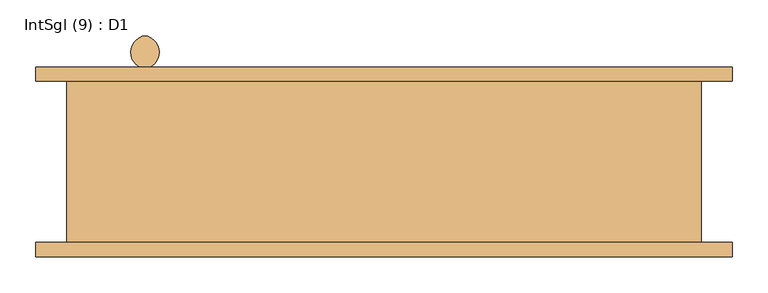
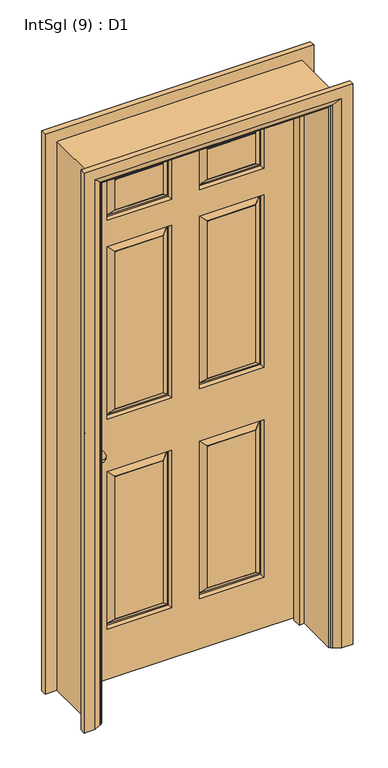
"""IFC4 building model written with IfcOpenShell, lengths in millimetres: door geometry, IntSgl (9) : D1."""

from ifc_helpers import new_model, si_unit, point, frame, origin, place, context, project, spatial, polyline, circle_curve, ellipse_curve, trimmed, outline, extrude, faceted_brep, source, transform, mapped, element, save
from ifc_brep_helpers import plane_surface, cylinder_surface, revolved_surface, advanced_brep


def intsgl_9_d1_c400c9dc(model_context):
    return source(origin(), model_context, "Body", "SolidModel", [
        advanced_brep(
        [(-328.0, 55.5, 900.0), (-333.0, 11.062589, 900.0), (-338.0, 55.5, 900.0), (-338.0, 70.5, 900.0), (-328.0, 70.5, 900.0), (-353.0, 74.5, 900.0), (-313.0, 74.5, 900.0), (-353.0, 70.5, 900.0), (-313.0, 70.5, 900.0)],
        [
            (0, 1, circle_curve(frame((-336.1884862, 33.9213505, 900.0), z_axis=(0.0, 0.0, -1.0), x_axis=(0.0, 1.0, 0.0)), 23.0800654)),
            (1, 2, circle_curve(frame((-329.8115138, 33.9213505, 900.0), z_axis=(0.0, 0.0, -1.0), x_axis=(0.0, 1.0, 0.0)), 23.0800654)),
            (2, 0, circle_curve(frame((-333.0, 55.5, 900.0), z_axis=(0.0, -1.0, 0.0), x_axis=(-1.0, 0.0, 0.0)), 5.0)),
            (0, 2, circle_curve(frame((-333.0, 55.5, 900.0), z_axis=(0.0, -1.0, 0.0), x_axis=(-1.0, 0.0, 0.0)), 5.0)),
            (2, 3),
            (3, 4, circle_curve(frame((-333.0, 70.5, 900.0), z_axis=(0.0, -1.0, 0.0), x_axis=(-1.0, 0.0, 0.0)), 5.0)),
            (4, 0),
            (4, 3, circle_curve(frame((-333.0, 70.5, 900.0), z_axis=(0.0, -1.0, 0.0), x_axis=(-1.0, 0.0, 0.0)), 5.0)),
            (5, 6, circle_curve(frame((-333.0, 74.5, 900.0), z_axis=(0.0, 1.0, 0.0), x_axis=(1.0, 0.0, 0.0)), 20.0)),
            (6, 5, circle_curve(frame((-333.0, 74.5, 900.0), z_axis=(0.0, 1.0, 0.0), x_axis=(1.0, 0.0, 0.0)), 20.0)),
            (7, 8, circle_curve(frame((-333.0, 70.5, 900.0), z_axis=(0.0, -1.0, 0.0), x_axis=(1.0, 0.0, 0.0)), 20.0)),
            (8, 7, circle_curve(frame((-333.0, 70.5, 900.0), z_axis=(0.0, -1.0, 0.0), x_axis=(1.0, 0.0, 0.0)), 20.0)),
            (6, 8),
            (7, 5),
        ],
        [
            revolved_surface(trimmed(ellipse_curve(frame((-329.8115138, 33.9213505, 900.0), z_axis=(0.0, 0.0, -1.0), x_axis=(0.0, 1.0, 0.0)), 23.0800654, 23.0800654), [point((-333.0, 11.062589, 900.0))], [point((-338.0, 55.5, 900.0))], True, "CARTESIAN"), (-333.0, 70.5, 900.0), (0.0, 1.0, 0.0)),
            cylinder_surface(frame((-333.0, 70.5, 900.0), z_axis=(0.0, 1.0, 0.0), x_axis=(-1.0, 0.0, 0.0)), 5.0),
            plane_surface(frame((-313.0, 74.5, 900.0), z_axis=(0.0, 1.0, 0.0), x_axis=(0.0, 0.0, 1.0))),
            plane_surface(frame((-313.0, 70.5, 900.0), z_axis=(0.0, -1.0, 0.0), x_axis=(0.0, 0.0, -1.0))),
            cylinder_surface(frame((-333.0, 70.5, 900.0), z_axis=(0.0, 1.0, 0.0), x_axis=(1.0, 0.0, 0.0)), 20.0),
        ],
        [
            (0, [[1, 2, 3]]),
            (0, [[-1, 4, -2]]),
            (1, [[5, 6, 7, -3]]),
            (1, [[-7, 8, -5, -4]]),
            (2, [[9, 10]]),
            (3, [[11, 12], [-8, -6]]),
            (4, [[13, -11, 14, -10]]),
            (4, [[-14, -12, -13, -9]]),
        ],
    ),
        advanced_brep(
        [(-328.0, 131.5, 900.0), (-338.0, 131.5, 900.0), (-333.0, 175.937411, 900.0), (-328.0, 116.5, 900.0), (-338.0, 116.5, 900.0), (-353.0, 112.5, 900.0), (-313.0, 112.5, 900.0), (-353.0, 116.5, 900.0), (-313.0, 116.5, 900.0)],
        [
            (0, 1, circle_curve(frame((-333.0, 131.5, 900.0), z_axis=(0.0, 1.0, 0.0), x_axis=(-1.0, 0.0, 0.0)), 5.0)),
            (1, 2, circle_curve(frame((-329.8115138, 153.0786495, 900.0), z_axis=(0.0, 0.0, -1.0), x_axis=(0.0, -1.0, 0.0)), 23.0800654)),
            (2, 0, circle_curve(frame((-336.1884862, 153.0786495, 900.0), z_axis=(0.0, 0.0, -1.0), x_axis=(0.0, -1.0, 0.0)), 23.0800654)),
            (1, 0, circle_curve(frame((-333.0, 131.5, 900.0), z_axis=(0.0, 1.0, 0.0), x_axis=(-1.0, 0.0, 0.0)), 5.0)),
            (0, 3),
            (3, 4, circle_curve(frame((-333.0, 116.5, 900.0), z_axis=(0.0, 1.0, 0.0), x_axis=(-1.0, 0.0, 0.0)), 5.0)),
            (4, 1),
            (4, 3, circle_curve(frame((-333.0, 116.5, 900.0), z_axis=(0.0, 1.0, 0.0), x_axis=(-1.0, 0.0, 0.0)), 5.0)),
            (5, 6, circle_curve(frame((-333.0, 112.5, 900.0), z_axis=(0.0, -1.0, 0.0), x_axis=(1.0, 0.0, 0.0)), 20.0)),
            (6, 5, circle_curve(frame((-333.0, 112.5, 900.0), z_axis=(0.0, -1.0, 0.0), x_axis=(1.0, 0.0, 0.0)), 20.0)),
            (7, 8, circle_curve(frame((-333.0, 116.5, 900.0), z_axis=(0.0, 1.0, 0.0), x_axis=(1.0, 0.0, 0.0)), 20.0)),
            (8, 7, circle_curve(frame((-333.0, 116.5, 900.0), z_axis=(0.0, 1.0, 0.0), x_axis=(1.0, 0.0, 0.0)), 20.0)),
            (5, 7),
            (8, 6),
        ],
        [
            revolved_surface(trimmed(ellipse_curve(frame((-329.8115138, 153.0786495, 900.0), z_axis=(0.0, 0.0, 1.0), x_axis=(0.0, -1.0, 0.0)), 23.0800654, 23.0800654), [point((-333.0, 175.937411, 900.0))], [point((-338.0, 131.5, 900.0))], True, "CARTESIAN"), (-333.0, 116.5, 900.0), (0.0, -1.0, 0.0)),
            cylinder_surface(frame((-333.0, 116.5, 900.0), z_axis=(0.0, -1.0, 0.0), x_axis=(-1.0, 0.0, 0.0)), 5.0),
            plane_surface(frame((-313.0, 112.5, 900.0), z_axis=(0.0, -1.0, 0.0), x_axis=(0.0, 0.0, 1.0))),
            plane_surface(frame((-313.0, 116.5, 900.0), z_axis=(0.0, 1.0, 0.0), x_axis=(0.0, 0.0, -1.0))),
            cylinder_surface(frame((-333.0, 116.5, 900.0), z_axis=(0.0, -1.0, 0.0), x_axis=(1.0, 0.0, 0.0)), 20.0),
        ],
        [
            (0, [[1, 2, 3]]),
            (0, [[-2, 4, -3]]),
            (1, [[-1, 5, 6, 7]]),
            (1, [[-4, -7, 8, -5]]),
            (2, [[9, 10]]),
            (3, [[11, 12], [-6, -8]]),
            (4, [[-9, 13, -12, 14]]),
            (4, [[-10, -14, -11, -13]]),
        ],
    ),
        faceted_brep([(-408.0, 74.5, 2058.0), (-408.0, 74.5, 8.0), (408.0, 74.5, 8.0), (408.0, 74.5, 2058.0), (-50.0, 74.5, 800.0), (-50.0, 74.5, 200.0), (-283.0, 74.5, 200.0), (-283.0, 74.5, 800.0), (283.0, 74.5, 800.0), (283.0, 74.5, 200.0), (50.0, 74.5, 200.0), (50.0, 74.5, 800.0), (-50.0, 74.5, 1658.0), (-50.0, 74.5, 1000.0), (-283.0, 74.5, 1000.0), (-283.0, 74.5, 1658.0), (283.0, 74.5, 1658.0), (283.0, 74.5, 1000.0), (50.0, 74.5, 1000.0), (50.0, 74.5, 1658.0), (-50.0, 74.5, 1933.0), (-50.0, 74.5, 1758.0), (-283.0, 74.5, 1758.0), (-283.0, 74.5, 1933.0), (283.0, 74.5, 1933.0), (283.0, 74.5, 1758.0), (50.0, 74.5, 1758.0), (50.0, 74.5, 1933.0), (-80.0, 74.5, 230.0), (-80.0, 74.5, 770.0), (-253.0, 74.5, 770.0), (-253.0, 74.5, 230.0), (253.0, 74.5, 230.0), (253.0, 74.5, 770.0), (80.0, 74.5, 770.0), (80.0, 74.5, 230.0), (-80.0, 74.5, 1030.0), (-80.0, 74.5, 1628.0), (-253.0, 74.5, 1628.0), (-253.0, 74.5, 1030.0), (253.0, 74.5, 1030.0), (253.0, 74.5, 1628.0), (80.0, 74.5, 1628.0), (80.0, 74.5, 1030.0), (-80.0, 74.5, 1788.0), (-80.0, 74.5, 1903.0), (-253.0, 74.5, 1903.0), (-253.0, 74.5, 1788.0), (253.0, 74.5, 1788.0), (253.0, 74.5, 1903.0), (80.0, 74.5, 1903.0), (80.0, 74.5, 1788.0), (-408.0, 112.5, 2058.0), (408.0, 112.5, 2058.0), (408.0, 112.5, 8.0), (-408.0, 112.5, 8.0), (50.0, 112.5, 800.0), (50.0, 112.5, 200.0), (283.0, 112.5, 200.0), (283.0, 112.5, 800.0), (-283.0, 112.5, 800.0), (-283.0, 112.5, 200.0), (-50.0, 112.5, 200.0), (-50.0, 112.5, 800.0), (50.0, 112.5, 1658.0), (50.0, 112.5, 1000.0), (283.0, 112.5, 1000.0), (283.0, 112.5, 1658.0), (-283.0, 112.5, 1658.0), (-283.0, 112.5, 1000.0), (-50.0, 112.5, 1000.0), (-50.0, 112.5, 1658.0), (50.0, 112.5, 1933.0), (50.0, 112.5, 1758.0), (283.0, 112.5, 1758.0), (283.0, 112.5, 1933.0), (-283.0, 112.5, 1933.0), (-283.0, 112.5, 1758.0), (-50.0, 112.5, 1758.0), (-50.0, 112.5, 1933.0), (80.0, 112.5, 230.0), (80.0, 112.5, 770.0), (253.0, 112.5, 770.0), (253.0, 112.5, 230.0), (-253.0, 112.5, 230.0), (-253.0, 112.5, 770.0), (-80.0, 112.5, 770.0), (-80.0, 112.5, 230.0), (80.0, 112.5, 1030.0), (80.0, 112.5, 1628.0), (253.0, 112.5, 1628.0), (253.0, 112.5, 1030.0), (-253.0, 112.5, 1030.0), (-253.0, 112.5, 1628.0), (-80.0, 112.5, 1628.0), (-80.0, 112.5, 1030.0), (80.0, 112.5, 1788.0), (80.0, 112.5, 1903.0), (253.0, 112.5, 1903.0), (253.0, 112.5, 1788.0), (-253.0, 112.5, 1788.0), (-253.0, 112.5, 1903.0), (-80.0, 112.5, 1903.0), (-80.0, 112.5, 1788.0), (80.0, 111.5, 230.0), (80.0, 111.5, 770.0), (58.0, 97.5, 208.0), (58.0, 97.5, 792.0), (78.0, 111.5, 772.0), (78.0, 111.5, 228.0), (53.0, 97.5, 797.0), (53.0, 97.5, 203.0), (253.0, 111.5, 770.0), (275.0, 97.5, 792.0), (255.0, 111.5, 772.0), (280.0, 97.5, 797.0), (253.0, 111.5, 230.0), (275.0, 97.5, 208.0), (255.0, 111.5, 228.0), (280.0, 97.5, 203.0), (-253.0, 111.5, 230.0), (-253.0, 111.5, 770.0), (-275.0, 97.5, 208.0), (-275.0, 97.5, 792.0), (-255.0, 111.5, 772.0), (-255.0, 111.5, 228.0), (-280.0, 97.5, 797.0), (-280.0, 97.5, 203.0), (-80.0, 111.5, 770.0), (-58.0, 97.5, 792.0), (-78.0, 111.5, 772.0), (-53.0, 97.5, 797.0), (-80.0, 111.5, 230.0), (-58.0, 97.5, 208.0), (-78.0, 111.5, 228.0), (-53.0, 97.5, 203.0), (80.0, 111.5, 1030.0), (80.0, 111.5, 1628.0), (58.0, 97.5, 1008.0), (58.0, 97.5, 1650.0), (78.0, 111.5, 1630.0), (78.0, 111.5, 1028.0), (53.0, 97.5, 1655.0), (53.0, 97.5, 1003.0), (253.0, 111.5, 1628.0), (275.0, 97.5, 1650.0), (255.0, 111.5, 1630.0), (280.0, 97.5, 1655.0), (253.0, 111.5, 1030.0), (275.0, 97.5, 1008.0), (255.0, 111.5, 1028.0), (280.0, 97.5, 1003.0), (-253.0, 111.5, 1030.0), (-253.0, 111.5, 1628.0), (-275.0, 97.5, 1008.0), (-275.0, 97.5, 1650.0), (-255.0, 111.5, 1630.0), (-255.0, 111.5, 1028.0), (-280.0, 97.5, 1655.0), (-280.0, 97.5, 1003.0), (-80.0, 111.5, 1628.0), (-58.0, 97.5, 1650.0), (-78.0, 111.5, 1630.0), (-53.0, 97.5, 1655.0), (-80.0, 111.5, 1030.0), (-58.0, 97.5, 1008.0), (-78.0, 111.5, 1028.0), (-53.0, 97.5, 1003.0), (80.0, 111.5, 1788.0), (80.0, 111.5, 1903.0), (58.0, 97.5, 1766.0), (58.0, 97.5, 1925.0), (78.0, 111.5, 1905.0), (78.0, 111.5, 1786.0), (53.0, 97.5, 1930.0), (53.0, 97.5, 1761.0), (253.0, 111.5, 1903.0), (275.0, 97.5, 1925.0), (255.0, 111.5, 1905.0), (280.0, 97.5, 1930.0), (253.0, 111.5, 1788.0), (275.0, 97.5, 1766.0), (255.0, 111.5, 1786.0), (280.0, 97.5, 1761.0), (-253.0, 111.5, 1788.0), (-253.0, 111.5, 1903.0), (-275.0, 97.5, 1766.0), (-275.0, 97.5, 1925.0), (-255.0, 111.5, 1905.0), (-255.0, 111.5, 1786.0), (-280.0, 97.5, 1930.0), (-280.0, 97.5, 1761.0), (-80.0, 111.5, 1903.0), (-58.0, 97.5, 1925.0), (-78.0, 111.5, 1905.0), (-53.0, 97.5, 1930.0), (-80.0, 111.5, 1788.0), (-58.0, 97.5, 1766.0), (-78.0, 111.5, 1786.0), (-53.0, 97.5, 1761.0), (-80.0, 75.5, 230.0), (-80.0, 75.5, 770.0), (-58.0, 89.5, 208.0), (-58.0, 89.5, 792.0), (-78.0, 75.5, 772.0), (-78.0, 75.5, 228.0), (-53.0, 89.5, 797.0), (-53.0, 89.5, 203.0), (-253.0, 75.5, 770.0), (-275.0, 89.5, 792.0), (-255.0, 75.5, 772.0), (-280.0, 89.5, 797.0), (-253.0, 75.5, 230.0), (-275.0, 89.5, 208.0), (-255.0, 75.5, 228.0), (-280.0, 89.5, 203.0), (253.0, 75.5, 230.0), (253.0, 75.5, 770.0), (275.0, 89.5, 208.0), (275.0, 89.5, 792.0), (255.0, 75.5, 772.0), (255.0, 75.5, 228.0), (280.0, 89.5, 797.0), (280.0, 89.5, 203.0), (80.0, 75.5, 770.0), (58.0, 89.5, 792.0), (78.0, 75.5, 772.0), (53.0, 89.5, 797.0), (80.0, 75.5, 230.0), (58.0, 89.5, 208.0), (78.0, 75.5, 228.0), (53.0, 89.5, 203.0), (-80.0, 75.5, 1030.0), (-80.0, 75.5, 1628.0), (-58.0, 89.5, 1008.0), (-58.0, 89.5, 1650.0), (-78.0, 75.5, 1630.0), (-78.0, 75.5, 1028.0), (-53.0, 89.5, 1655.0), (-53.0, 89.5, 1003.0), (-253.0, 75.5, 1628.0), (-275.0, 89.5, 1650.0), (-255.0, 75.5, 1630.0), (-280.0, 89.5, 1655.0), (-253.0, 75.5, 1030.0), (-275.0, 89.5, 1008.0), (-255.0, 75.5, 1028.0), (-280.0, 89.5, 1003.0), (253.0, 75.5, 1030.0), (253.0, 75.5, 1628.0), (275.0, 89.5, 1008.0), (275.0, 89.5, 1650.0), (255.0, 75.5, 1630.0), (255.0, 75.5, 1028.0), (280.0, 89.5, 1655.0), (280.0, 89.5, 1003.0), (80.0, 75.5, 1628.0), (58.0, 89.5, 1650.0), (78.0, 75.5, 1630.0), (53.0, 89.5, 1655.0), (80.0, 75.5, 1030.0), (58.0, 89.5, 1008.0), (78.0, 75.5, 1028.0), (53.0, 89.5, 1003.0), (-80.0, 75.5, 1788.0), (-80.0, 75.5, 1903.0), (-58.0, 89.5, 1766.0), (-58.0, 89.5, 1925.0), (-78.0, 75.5, 1905.0), (-78.0, 75.5, 1786.0), (-53.0, 89.5, 1930.0), (-53.0, 89.5, 1761.0), (-253.0, 75.5, 1903.0), (-275.0, 89.5, 1925.0), (-255.0, 75.5, 1905.0), (-280.0, 89.5, 1930.0), (-253.0, 75.5, 1788.0), (-275.0, 89.5, 1766.0), (-255.0, 75.5, 1786.0), (-280.0, 89.5, 1761.0), (253.0, 75.5, 1788.0), (253.0, 75.5, 1903.0), (275.0, 89.5, 1766.0), (275.0, 89.5, 1925.0), (255.0, 75.5, 1905.0), (255.0, 75.5, 1786.0), (280.0, 89.5, 1930.0), (280.0, 89.5, 1761.0), (80.0, 75.5, 1903.0), (58.0, 89.5, 1925.0), (78.0, 75.5, 1905.0), (53.0, 89.5, 1930.0), (80.0, 75.5, 1788.0), (58.0, 89.5, 1766.0), (78.0, 75.5, 1786.0), (53.0, 89.5, 1761.0)], [[[0, 1, 2, 3], [4, 5, 6, 7], [8, 9, 10, 11], [12, 13, 14, 15], [16, 17, 18, 19], [20, 21, 22, 23], [24, 25, 26, 27]], [[28, 29, 30, 31]], [[32, 33, 34, 35]], [[36, 37, 38, 39]], [[40, 41, 42, 43]], [[44, 45, 46, 47]], [[48, 49, 50, 51]], [[52, 53, 54, 55], [56, 57, 58, 59], [60, 61, 62, 63], [64, 65, 66, 67], [68, 69, 70, 71], [72, 73, 74, 75], [76, 77, 78, 79]], [[80, 81, 82, 83]], [[84, 85, 86, 87]], [[88, 89, 90, 91]], [[92, 93, 94, 95]], [[96, 97, 98, 99]], [[100, 101, 102, 103]], [[1, 0, 52, 55]], [[2, 1, 55, 54]], [[3, 2, 54, 53]], [[0, 3, 53, 52]], [[104, 105, 81, 80]], [[106, 107, 108, 109]], [[56, 110, 111, 57]], [[81, 105, 112, 82]], [[108, 107, 113, 114]], [[110, 56, 59, 115]], [[82, 112, 116, 83]], [[114, 113, 117, 118]], [[115, 59, 58, 119]], [[104, 80, 83, 116]], [[109, 108, 114, 118], [105, 104, 116, 112]], [[106, 109, 118, 117]], [[111, 110, 115, 119], [107, 106, 117, 113]], [[57, 111, 119, 58]], [[120, 121, 85, 84]], [[122, 123, 124, 125]], [[60, 126, 127, 61]], [[85, 121, 128, 86]], [[124, 123, 129, 130]], [[126, 60, 63, 131]], [[86, 128, 132, 87]], [[130, 129, 133, 134]], [[131, 63, 62, 135]], [[120, 84, 87, 132]], [[125, 124, 130, 134], [121, 120, 132, 128]], [[122, 125, 134, 133]], [[127, 126, 131, 135], [123, 122, 133, 129]], [[61, 127, 135, 62]], [[136, 137, 89, 88]], [[138, 139, 140, 141]], [[64, 142, 143, 65]], [[89, 137, 144, 90]], [[140, 139, 145, 146]], [[142, 64, 67, 147]], [[90, 144, 148, 91]], [[146, 145, 149, 150]], [[147, 67, 66, 151]], [[136, 88, 91, 148]], [[141, 140, 146, 150], [137, 136, 148, 144]], [[138, 141, 150, 149]], [[143, 142, 147, 151], [139, 138, 149, 145]], [[65, 143, 151, 66]], [[152, 153, 93, 92]], [[154, 155, 156, 157]], [[68, 158, 159, 69]], [[93, 153, 160, 94]], [[156, 155, 161, 162]], [[158, 68, 71, 163]], [[94, 160, 164, 95]], [[162, 161, 165, 166]], [[163, 71, 70, 167]], [[152, 92, 95, 164]], [[157, 156, 162, 166], [153, 152, 164, 160]], [[154, 157, 166, 165]], [[159, 158, 163, 167], [155, 154, 165, 161]], [[69, 159, 167, 70]], [[168, 169, 97, 96]], [[170, 171, 172, 173]], [[72, 174, 175, 73]], [[97, 169, 176, 98]], [[172, 171, 177, 178]], [[174, 72, 75, 179]], [[98, 176, 180, 99]], [[178, 177, 181, 182]], [[179, 75, 74, 183]], [[168, 96, 99, 180]], [[173, 172, 178, 182], [169, 168, 180, 176]], [[170, 173, 182, 181]], [[175, 174, 179, 183], [171, 170, 181, 177]], [[73, 175, 183, 74]], [[184, 185, 101, 100]], [[186, 187, 188, 189]], [[76, 190, 191, 77]], [[101, 185, 192, 102]], [[188, 187, 193, 194]], [[190, 76, 79, 195]], [[102, 192, 196, 103]], [[194, 193, 197, 198]], [[195, 79, 78, 199]], [[184, 100, 103, 196]], [[189, 188, 194, 198], [185, 184, 196, 192]], [[186, 189, 198, 197]], [[191, 190, 195, 199], [187, 186, 197, 193]], [[77, 191, 199, 78]], [[200, 201, 29, 28]], [[202, 203, 204, 205]], [[4, 206, 207, 5]], [[29, 201, 208, 30]], [[204, 203, 209, 210]], [[206, 4, 7, 211]], [[30, 208, 212, 31]], [[210, 209, 213, 214]], [[211, 7, 6, 215]], [[200, 28, 31, 212]], [[205, 204, 210, 214], [201, 200, 212, 208]], [[202, 205, 214, 213]], [[207, 206, 211, 215], [203, 202, 213, 209]], [[5, 207, 215, 6]], [[216, 217, 33, 32]], [[218, 219, 220, 221]], [[8, 222, 223, 9]], [[33, 217, 224, 34]], [[220, 219, 225, 226]], [[222, 8, 11, 227]], [[34, 224, 228, 35]], [[226, 225, 229, 230]], [[227, 11, 10, 231]], [[216, 32, 35, 228]], [[221, 220, 226, 230], [217, 216, 228, 224]], [[218, 221, 230, 229]], [[223, 222, 227, 231], [219, 218, 229, 225]], [[9, 223, 231, 10]], [[232, 233, 37, 36]], [[234, 235, 236, 237]], [[12, 238, 239, 13]], [[37, 233, 240, 38]], [[236, 235, 241, 242]], [[238, 12, 15, 243]], [[38, 240, 244, 39]], [[242, 241, 245, 246]], [[243, 15, 14, 247]], [[232, 36, 39, 244]], [[237, 236, 242, 246], [233, 232, 244, 240]], [[234, 237, 246, 245]], [[239, 238, 243, 247], [235, 234, 245, 241]], [[13, 239, 247, 14]], [[248, 249, 41, 40]], [[250, 251, 252, 253]], [[16, 254, 255, 17]], [[41, 249, 256, 42]], [[252, 251, 257, 258]], [[254, 16, 19, 259]], [[42, 256, 260, 43]], [[258, 257, 261, 262]], [[259, 19, 18, 263]], [[248, 40, 43, 260]], [[253, 252, 258, 262], [249, 248, 260, 256]], [[250, 253, 262, 261]], [[255, 254, 259, 263], [251, 250, 261, 257]], [[17, 255, 263, 18]], [[264, 265, 45, 44]], [[266, 267, 268, 269]], [[20, 270, 271, 21]], [[45, 265, 272, 46]], [[268, 267, 273, 274]], [[270, 20, 23, 275]], [[46, 272, 276, 47]], [[274, 273, 277, 278]], [[275, 23, 22, 279]], [[264, 44, 47, 276]], [[269, 268, 274, 278], [265, 264, 276, 272]], [[266, 269, 278, 277]], [[271, 270, 275, 279], [267, 266, 277, 273]], [[21, 271, 279, 22]], [[280, 281, 49, 48]], [[282, 283, 284, 285]], [[24, 286, 287, 25]], [[49, 281, 288, 50]], [[284, 283, 289, 290]], [[286, 24, 27, 291]], [[50, 288, 292, 51]], [[290, 289, 293, 294]], [[291, 27, 26, 295]], [[280, 48, 51, 292]], [[285, 284, 290, 294], [281, 280, 292, 288]], [[282, 285, 294, 293]], [[287, 286, 291, 295], [283, 282, 293, 289]], [[25, 287, 295, 26]]]),
        faceted_brep([(-410.0, 112.5, 0.0), (-410.0, -112.5, 0.0), (-442.0, -112.5, 0.0), (-442.0, 112.5, 0.0), (-410.0, 112.5, 2060.0), (-410.0, -112.5, 2060.0), (-442.0, -112.5, 2092.0), (-442.0, 112.5, 2092.0), (410.0, 112.5, 0.0), (442.0, 112.5, 0.0), (442.0, -112.5, 0.0), (410.0, -112.5, 0.0), (410.0, 112.5, 2060.0), (442.0, 112.5, 2092.0), (442.0, -112.5, 2092.0), (410.0, -112.5, 2060.0)], [[[0, 1, 2, 3]], [[1, 0, 4, 5]], [[2, 1, 5, 6]], [[3, 2, 6, 7]], [[0, 3, 7, 4]], [[8, 9, 10, 11]], [[12, 13, 9, 8]], [[13, 14, 10, 9]], [[14, 15, 11, 10]], [[15, 12, 8, 11]], [[5, 4, 12, 15]], [[6, 5, 15, 14]], [[7, 6, 14, 13]], [[4, 7, 13, 12]]]),
        extrude(outline(polyline([(0.0, -410.0), (0.0, -391.0), (2041.0, -391.0), (2041.0, 391.0), (0.0, 391.0), (0.0, 410.0), (2060.0, 410.0), (2060.0, -410.0), (0.0, -410.0)])), frame((0.0, 40.5, 0.0), z_axis=(0.0, 1.0, 0.0), x_axis=(0.0, 0.0, 1.0)), (0.0, 0.0, 1.0), 32.0),
        advanced_brep(
        [(-485.0, -132.5, 0.0), (-485.0, -112.5, 0.0), (-415.0, -112.5, 0.0), (-419.0, -118.5, 0.0), (-445.0, -132.5, 0.0), (-485.0, -132.5, 2135.0), (-485.0, -112.5, 2135.0), (485.0, -112.5, 2135.0), (485.0, -112.5, 0.0), (415.0, -112.5, 0.0), (415.0, -112.5, 2065.0), (-415.0, -112.5, 2065.0), (-419.0, -118.5, 2069.0), (-445.0, -132.5, 2095.0), (445.0, -132.5, 2095.0), (445.0, -132.5, 0.0), (485.0, -132.5, 0.0), (485.0, -132.5, 2135.0), (419.0, -118.5, 0.0), (419.0, -118.5, 2069.0)],
        [
            (0, 1),
            (1, 2),
            (2, 3, circle_curve(frame((-423.0, -111.5, 0.0), z_axis=(0.0, 0.0, -1.0), x_axis=(-1.0, 0.0, 0.0)), 8.0622577)),
            (3, 4),
            (4, 0),
            (0, 5),
            (5, 6),
            (6, 1),
            (6, 7),
            (7, 8),
            (8, 9),
            (9, 10),
            (10, 11),
            (11, 2),
            (11, 12, ellipse_curve(frame((-423.0, -111.5, 2073.0), z_axis=(-0.7071067811865475, 0.0, -0.7071067811865475), x_axis=(0.7071067811865474, 0.0, -0.7071067811865476)), 11.4017543, 8.0622577)),
            (12, 3),
            (12, 13),
            (13, 4),
            (13, 14),
            (14, 15),
            (15, 16),
            (16, 17),
            (17, 5),
            (7, 17),
            (16, 8),
            (15, 18),
            (18, 9, circle_curve(frame((423.0, -111.5, 0.0), z_axis=(0.0, 0.0, -1.0), x_axis=(1.0, 0.0, 0.0)), 8.0622577)),
            (19, 10, ellipse_curve(frame((423.0, -111.5, 2073.0), z_axis=(0.7071067811865475, 0.0, -0.7071067811865475), x_axis=(0.7071067811865474, 0.0, 0.7071067811865476)), 11.4017543, 8.0622577)),
            (18, 19),
            (14, 19),
            (19, 12),
        ],
        [
            plane_surface(frame((-415.0, -112.5, 0.0), z_axis=(0.0, 0.0, -1.0), x_axis=(0.0, -1.0, 0.0))),
            plane_surface(frame((-485.0, -132.5, 0.0), z_axis=(-1.0, 0.0, 0.0), x_axis=(0.0, 0.0, 1.0))),
            plane_surface(frame((-485.0, -112.5, 0.0), z_axis=(0.0, 1.0, 0.0), x_axis=(0.0, 0.0, 1.0))),
            cylinder_surface(frame((-423.0, -111.5, 0.0), z_axis=(0.0, 0.0, -1.0), x_axis=(-1.0, 0.0, 0.0)), 8.0622577),
            plane_surface(frame((-419.0, -118.5, 0.0), z_axis=(0.4740998230350183, -0.8804710999221749, 0.0), x_axis=(0.0, 0.0, 1.0))),
            plane_surface(frame((-445.0, -132.5, 0.0), z_axis=(0.0, -1.0, 0.0), x_axis=(0.0, 0.0, 1.0))),
            plane_surface(frame((485.0, -132.5, 2135.0), z_axis=(1.0, 0.0, 0.0), x_axis=(0.0, 0.0, -1.0))),
            plane_surface(frame((415.0, -112.5, 0.0), z_axis=(0.0, 0.0, -1.0), x_axis=(0.0, -1.0, 0.0))),
            cylinder_surface(frame((423.0, -111.5, 2065.0), z_axis=(0.0, 0.0, 1.0), x_axis=(1.0, 0.0, 0.0)), 8.0622577),
            plane_surface(frame((419.0, -118.5, 2069.0), z_axis=(-0.4740998230350183, -0.8804710999221749, 0.0), x_axis=(0.0, 0.0, -1.0))),
            plane_surface(frame((-485.0, -132.5, 2135.0), z_axis=(0.0, 0.0, 1.0), x_axis=(1.0, 0.0, 0.0))),
            cylinder_surface(frame((-415.0, -111.5, 2073.0), z_axis=(-1.0, 0.0, 0.0), x_axis=(0.0, 0.0, 1.0)), 8.0622577),
            plane_surface(frame((-419.0, -118.5, 2069.0), z_axis=(0.0, -0.8804710999221749, -0.4740998230350183), x_axis=(1.0, 0.0, 0.0))),
        ],
        [
            (0, [[1, 2, 3, 4, 5]]),
            (1, [[-1, 6, 7, 8]]),
            (2, [[-2, -8, 9, 10, 11, 12, 13, 14]]),
            (3, [[-3, -14, 15, 16]]),
            (4, [[-4, -16, 17, 18]]),
            (5, [[-5, -18, 19, 20, 21, 22, 23, -6]]),
            (6, [[24, -22, 25, -10]]),
            (7, [[-21, 26, 27, -11, -25]]),
            (8, [[28, -12, -27, 29]]),
            (9, [[30, -29, -26, -20]]),
            (10, [[-7, -23, -24, -9]]),
            (11, [[-15, -13, -28, 31]]),
            (12, [[-17, -31, -30, -19]]),
        ],
    ),
        advanced_brep(
        [(485.0, 132.5, 0.0), (485.0, 112.5, 0.0), (415.0, 112.5, 0.0), (419.0, 118.5, 0.0), (445.0, 132.5, 0.0), (485.0, 132.5, 2135.0), (485.0, 112.5, 2135.0), (-485.0, 112.5, 2135.0), (-485.0, 112.5, 0.0), (-415.0, 112.5, 0.0), (-415.0, 112.5, 2065.0), (415.0, 112.5, 2065.0), (419.0, 118.5, 2069.0), (445.0, 132.5, 2095.0), (-445.0, 132.5, 2095.0), (-445.0, 132.5, 0.0), (-485.0, 132.5, 0.0), (-485.0, 132.5, 2135.0), (-419.0, 118.5, 0.0), (-419.0, 118.5, 2069.0)],
        [
            (0, 1),
            (1, 2),
            (2, 3, circle_curve(frame((423.0, 111.5, 0.0), z_axis=(0.0, 0.0, -1.0), x_axis=(1.0, 0.0, 0.0)), 8.0622577)),
            (3, 4),
            (4, 0),
            (0, 5),
            (5, 6),
            (6, 1),
            (6, 7),
            (7, 8),
            (8, 9),
            (9, 10),
            (10, 11),
            (11, 2),
            (11, 12, ellipse_curve(frame((423.0, 111.5, 2073.0), z_axis=(0.7071067811865475, 0.0, -0.7071067811865475), x_axis=(-0.7071067811865474, 0.0, -0.7071067811865476)), 11.4017543, 8.0622577)),
            (12, 3),
            (12, 13),
            (13, 4),
            (13, 14),
            (14, 15),
            (15, 16),
            (16, 17),
            (17, 5),
            (7, 17),
            (16, 8),
            (15, 18),
            (18, 9, circle_curve(frame((-423.0, 111.5, 0.0), z_axis=(0.0, 0.0, -1.0), x_axis=(-1.0, 0.0, 0.0)), 8.0622577)),
            (19, 10, ellipse_curve(frame((-423.0, 111.5, 2073.0), z_axis=(-0.7071067811865475, 0.0, -0.7071067811865475), x_axis=(-0.7071067811865474, 0.0, 0.7071067811865476)), 11.4017543, 8.0622577)),
            (18, 19),
            (14, 19),
            (19, 12),
        ],
        [
            plane_surface(frame((415.0, 112.5, 0.0), z_axis=(0.0, 0.0, -1.0), x_axis=(0.0, 1.0, 0.0))),
            plane_surface(frame((485.0, 132.5, 0.0), z_axis=(1.0, 0.0, 0.0), x_axis=(0.0, 0.0, 1.0))),
            plane_surface(frame((485.0, 112.5, 0.0), z_axis=(0.0, -1.0, 0.0), x_axis=(0.0, 0.0, 1.0))),
            cylinder_surface(frame((423.0, 111.5, 0.0), z_axis=(0.0, 0.0, -1.0), x_axis=(1.0, 0.0, 0.0)), 8.0622577),
            plane_surface(frame((419.0, 118.5, 0.0), z_axis=(-0.4740998230350183, 0.8804710999221749, 0.0), x_axis=(0.0, 0.0, 1.0))),
            plane_surface(frame((445.0, 132.5, 0.0), z_axis=(0.0, 1.0, 0.0), x_axis=(0.0, 0.0, 1.0))),
            plane_surface(frame((-485.0, 132.5, 2135.0), z_axis=(-1.0, 0.0, 0.0), x_axis=(0.0, 0.0, -1.0))),
            plane_surface(frame((-415.0, 112.5, 0.0), z_axis=(0.0, 0.0, -1.0), x_axis=(0.0, 1.0, 0.0))),
            cylinder_surface(frame((-423.0, 111.5, 2065.0), z_axis=(0.0, 0.0, 1.0), x_axis=(-1.0, 0.0, 0.0)), 8.0622577),
            plane_surface(frame((-419.0, 118.5, 2069.0), z_axis=(0.4740998230350183, 0.8804710999221749, 0.0), x_axis=(0.0, 0.0, -1.0))),
            plane_surface(frame((485.0, 132.5, 2135.0), z_axis=(0.0, 0.0, 1.0), x_axis=(-1.0, 0.0, 0.0))),
            cylinder_surface(frame((415.0, 111.5, 2073.0), z_axis=(1.0, 0.0, 0.0), x_axis=(0.0, 0.0, 1.0)), 8.0622577),
            plane_surface(frame((419.0, 118.5, 2069.0), z_axis=(0.0, 0.8804710999221749, -0.4740998230350183), x_axis=(-1.0, 0.0, 0.0))),
        ],
        [
            (0, [[1, 2, 3, 4, 5]]),
            (1, [[-1, 6, 7, 8]]),
            (2, [[-2, -8, 9, 10, 11, 12, 13, 14]]),
            (3, [[-3, -14, 15, 16]]),
            (4, [[-4, -16, 17, 18]]),
            (5, [[-5, -18, 19, 20, 21, 22, 23, -6]]),
            (6, [[24, -22, 25, -10]]),
            (7, [[-21, 26, 27, -11, -25]]),
            (8, [[28, -12, -27, 29]]),
            (9, [[30, -29, -26, -20]]),
            (10, [[-7, -23, -24, -9]]),
            (11, [[-15, -13, -28, 31]]),
            (12, [[-17, -31, -30, -19]]),
        ],
    ),
    ])


if __name__ == "__main__":
    model = new_model("IFC4")
    model_context = context("Model", 3, world=origin())
    ifc_project = project(units=[si_unit("LENGTHUNIT", "METRE", prefix="MILLI")], contexts=[model_context])
    site = spatial("IfcSite", under=ifc_project)
    building = spatial("IfcBuilding", under=site)
    placement = place(None, origin())
    intsgl_9_d1_shape = intsgl_9_d1_c400c9dc(model_context)
    element("IfcDoor", 1, ObjectType="IntSgl (9) : D1", at=placement, inside=building, context=model_context, shape_type="MappedRepresentation", body=[
        mapped(intsgl_9_d1_shape, transform((0.0, 0.0, 0.0), x_axis=(1.0, 0.0, 0.0), y_axis=(0.0, 1.0, 0.0), z_axis=(0.0, 0.0, 1.0))),
    ])
    save(model, "model.ifc")

# Revit data of these elements
# Type "IntSgl (9) : D1"
#   Type Mark = "46"
#   Operation = "SingleSwingRight"
#   Manufacturer = "Revit"
#   Keynote = "L20"
#   UnderCut = 8 mm
#   Tolerance = 2 mm
#   Thickness = 38 mm
#   Structural Tolerance = 8 mm
#   StopDepth = 32 mm
#   Stop Thickness = 19 mm
#   Stile Top Rail = 125 mm
#   Stile Shutting = 125 mm
#   Stile Muntin Rail = 100 mm
#   Stile Lock Rail = 200 mm
#   Stile Intermediate/Frieze = 100 mm
#   Stile Hanging = 125 mm
#   Stile Bottom Rail = 200 mm
#   Rough Width = 900 mm
#   Rough Height = 2100 mm
#   Height to Top Lock Rail = 1000 mm
#   Handle Z Distance = 900 mm
#   Handle X Distance = 75 mm
#   Frame Thickness = 32 mm
#   Door Panel Width = 816 mm
#   Height = 2100 mm
#   Width = 900 mm
#   Door Panel Thickness = 38 mm
#   Door Panel Offset = 0 mm
#   Door Panel Height = 2050 mm
#   Architrave Setback = 5 mm
#   Vis - Ironmongery = yes
#   Material Ironmongery = Door - Handle
#   Material Frame = Door - Frame/Mullion
#   Material Door = Door - Panel
#   Material Architrave = Door - Architrave
#   Function = (empty or 0)
#   Wall Closure = (empty or 0)
# Element 1 (IfcDoor, "IntSgl (9) : D1")
#   Materials on its faces: "Door - Panel", "Door - Architrave", "Door - Frame/Mullion", "Door - Handle"
# Materials
#   "Door - Handle": colour RGB 247 247 247, transparency 0
#   "Door - Frame/Mullion": colour RGB 212 179 113, transparency 0
#   "Door - Panel": colour RGB 154 90 5, transparency 0
#   "Door - Architrave": colour RGB 154 90 5, transparency 0
